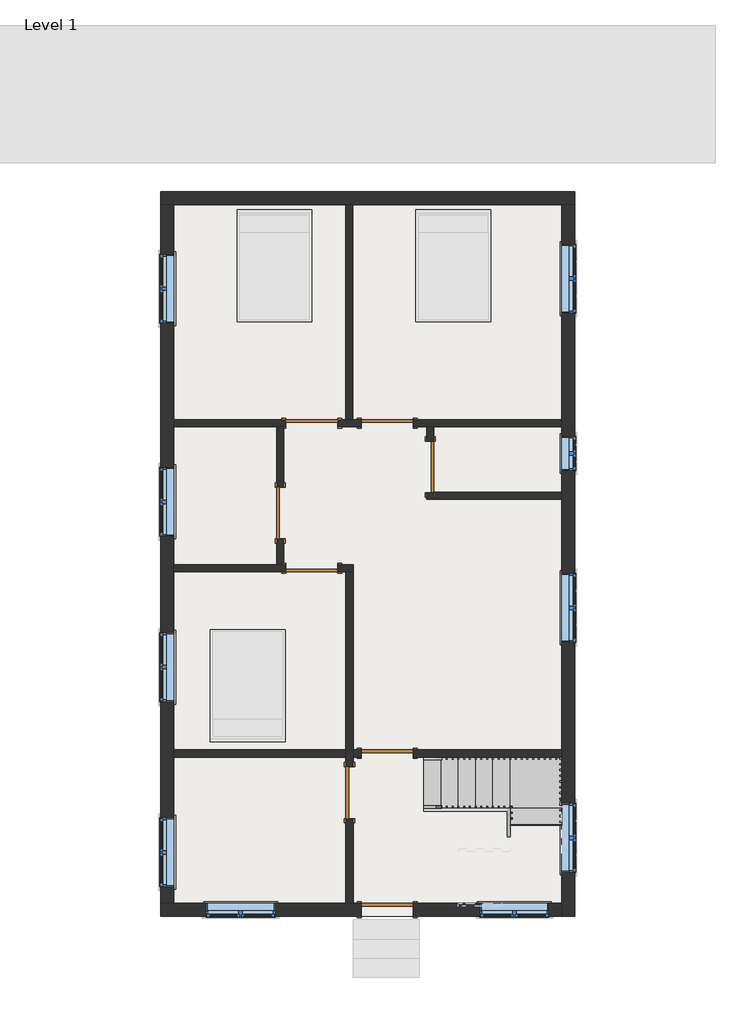
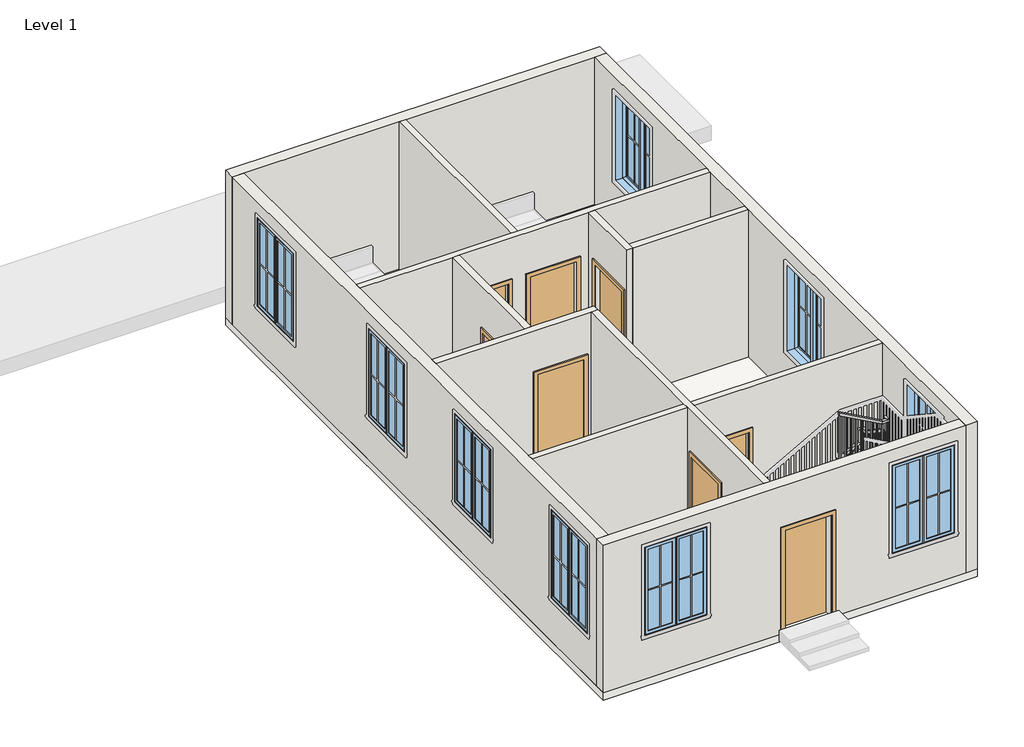
# One storey, part 1 of 2: 12 walls, 10 windows, 8 doors, 1 railing, 1 slab, 1 stair flight.
"""IFC4 building model written with IfcOpenShell, lengths in millimetres."""

from ifc_helpers import new_model, si_unit, frame, origin, origin_with_axes, place, context, project, spatial, polyline, outline, extrude, faceted_brep, transform, mapped, element, save
from components import door_a1797ceb, door_a3eb833a, door_a90ba1ad, stair_flight_16d52fd2, window_c417fced, window_6ca1769e

model = new_model("IFC4")

# Units and contexts
model_context = context("Model", 3, world=origin())
ifc_project = project(units=[si_unit("LENGTHUNIT", "METRE", prefix="MILLI")], contexts=[model_context])

# Site, building, storey
site = spatial("IfcSite", under=ifc_project)
building = spatial("IfcBuilding", under=site)
storey = spatial("IfcBuildingStorey", under=building, Name="Level 1", Elevation=0.0)

# Doors
placement = place(None, origin())
door_shape = door_a1797ceb(model_context)
element("IfcDoor", 1, ObjectType="Single-Flush : 36\" x 84\"", at=placement, inside=storey, context=model_context, shape_type="MappedRepresentation", body=[
    mapped(door_shape, transform((3683.0, 10363.2, 0.0), x_axis=(1.0, 0.0, 0.0), y_axis=(0.0, 1.0, 0.0), z_axis=(0.0, 0.0, 1.0))),
])
element("IfcDoor", 2, ObjectType="Single-Flush : 36\" x 84\"", at=placement, inside=storey, context=model_context, shape_type="MappedRepresentation", body=[
    mapped(door_shape, transform((3124.2, 8775.7, 0.0), x_axis=(0.0, 1.0, 0.0), y_axis=(-1.0, 0.0, 0.0), z_axis=(0.0, 0.0, 1.0))),
])
element("IfcDoor", 3, ObjectType="Single-Flush : 36\" x 84\"", at=placement, inside=storey, context=model_context, shape_type="MappedRepresentation", body=[
    mapped(door_shape, transform((3683.0, 7797.8, 0.0), x_axis=(-1.0, 0.0, 0.0), y_axis=(0.0, -1.0, 0.0), z_axis=(0.0, 0.0, 1.0))),
])
element("IfcDoor", 4, ObjectType="Single-Flush : 36\" x 84\"", at=placement, inside=storey, context=model_context, shape_type="MappedRepresentation", body=[
    mapped(door_shape, transform((4349.75, 3835.4, 0.0), x_axis=(0.0, 1.0, 0.0), y_axis=(-1.0, 0.0, 0.0), z_axis=(0.0, 0.0, 1.0))),
])
door_2_shape = door_a3eb833a(model_context)
element("IfcDoor", 5, ObjectType="Single-Flush : 36\" x 84\"", at=placement, inside=storey, context=model_context, shape_type="MappedRepresentation", body=[
    mapped(door_2_shape, transform((5016.5, 10363.2, 0.0), x_axis=(-1.0, 0.0, 0.0), y_axis=(0.0, -1.0, 0.0), z_axis=(0.0, 0.0, 1.0))),
])
element("IfcDoor", 6, ObjectType="Single-Flush : 36\" x 84\"", at=placement, inside=storey, context=model_context, shape_type="MappedRepresentation", body=[
    mapped(door_2_shape, transform((5778.5, 9588.5, 0.0), x_axis=(0.0, 1.0, 0.0), y_axis=(-1.0, 0.0, 0.0), z_axis=(0.0, 0.0, 1.0))),
])
element("IfcDoor", 7, ObjectType="Single-Flush : 36\" x 84\"", at=placement, inside=storey, context=model_context, shape_type="MappedRepresentation", body=[
    mapped(door_2_shape, transform((5016.5, 4527.55, 0.0), x_axis=(-1.0, 0.0, 0.0), y_axis=(0.0, -1.0, 0.0), z_axis=(0.0, 0.0, 1.0))),
])
door_3_shape = door_a90ba1ad(model_context)
element("IfcDoor", 8, ObjectType="Single-Flush : 36\" x 84\"", at=placement, inside=storey, context=model_context, shape_type="MappedRepresentation", body=[
    mapped(door_3_shape, transform((5016.5, 1765.3, 0.0), x_axis=(-1.0, 0.0, 0.0), y_axis=(0.0, -1.0, 0.0), z_axis=(0.0, 0.0, 1.0))),
])

# Railing
element("IfcRailing", 9, ObjectType="Handrail - Rectangular", at=placement, inside=storey, context=model_context, shape_type="SolidModel", body=[
    faceted_brep([(5664.2, 3606.8, 1083.7333333), (5664.2, 3606.8, 1025.620221), (5664.2, 3556.0, 1025.620221), (5664.2, 3556.0, 1083.7333333), (7112.0, 3606.8, 1888.0666667), (7162.8, 3606.8, 1858.1757765), (7162.8, 3556.0, 1858.1757765), (7112.0, 3556.0, 1888.0666667), (7112.0, 3606.8, 2150.5333333), (7162.8, 3606.8, 2099.7333333), (7162.8, 3556.0, 2099.7333333), (7112.0, 3556.0, 2150.5333333), (7239.0, 3606.8, 2150.5333333), (7239.0, 3606.8, 2099.7333333), (7188.2, 3556.0, 2099.7333333), (7188.2, 3556.0, 2150.5333333), (7239.0, 3479.8, 2150.5333333), (7239.0, 3464.4189976, 2099.7333333), (7188.2, 3464.4189976, 2099.7333333), (7188.2, 3479.8, 2150.5333333), (7239.0, 2870.2, 2556.9333333), (7239.0, 2819.4, 2529.7459984), (7188.2, 2819.4, 2529.7459984), (7188.2, 2870.2, 2556.9333333), (7239.0, 2870.2, 2819.3694921), (7239.0, 2819.4, 2768.5694921), (7188.2, 2819.4, 2768.5694921), (7188.2, 2870.2, 2819.3694921), (7239.0, 2743.2, 2819.3694921), (7239.0, 2743.2, 2768.5694921), (7188.2, 2794.0, 2768.5694921), (7188.2, 2794.0, 2819.3694921), (7112.0, 2743.2, 2819.3694921), (7098.8446915, 2743.2, 2768.5694921), (7098.8446915, 2794.0, 2768.5694921), (7112.0, 2794.0, 2819.3694921), (6273.1405542, 2743.2, 3285.0666667), (6273.1405542, 2794.0, 3285.0666667), (6273.1405542, 2794.0, 3226.9634289), (6273.1405542, 2743.2, 3226.9634289)], [[[0, 1, 2, 3]], [[1, 0, 4, 5]], [[2, 1, 5, 6]], [[3, 2, 6, 7]], [[0, 3, 7, 4]], [[5, 4, 8, 9]], [[6, 5, 9, 10]], [[7, 6, 10, 11]], [[4, 7, 11, 8]], [[9, 8, 12, 13]], [[10, 9, 13, 14]], [[11, 10, 14, 15]], [[8, 11, 15, 12]], [[13, 12, 16, 17]], [[14, 13, 17, 18]], [[15, 14, 18, 19]], [[12, 15, 19, 16]], [[17, 16, 20, 21]], [[18, 17, 21, 22]], [[19, 18, 22, 23]], [[16, 19, 23, 20]], [[21, 20, 24, 25]], [[22, 21, 25, 26]], [[23, 22, 26, 27]], [[20, 23, 27, 24]], [[25, 24, 28, 29]], [[26, 25, 29, 30]], [[27, 26, 30, 31]], [[24, 27, 31, 28]], [[29, 28, 32, 33]], [[30, 29, 33, 34]], [[31, 30, 34, 35]], [[28, 31, 35, 32]], [[36, 37, 38, 39]], [[33, 32, 36, 39]], [[34, 33, 39, 38]], [[35, 34, 38, 37]], [[32, 35, 37, 36]]]),
    extrude(outline(polyline([(3207.2085391, 6308.725), (3217.7842455, 6289.675), (2201.3333333, 6289.675), (2201.3333333, 6308.725), (3207.2085391, 6308.725)])), frame((0.0, 2759.075, 0.0), z_axis=(0.0, 1.0, 0.0), x_axis=(0.0, 0.0, 1.0)), (0.0, 0.0, 1.0), 19.05),
    extrude(outline(polyline([(3150.8047719, 6410.325), (3161.3804782, 6391.275), (2201.3333333, 6391.275), (2201.3333333, 6410.325), (3150.8047719, 6410.325)])), frame((0.0, 2759.075, 0.0), z_axis=(0.0, 1.0, 0.0), x_axis=(0.0, 0.0, 1.0)), (0.0, 0.0, 1.0), 19.05),
    extrude(outline(polyline([(3094.4010046, 6511.925), (3104.976711, 6492.875), (2201.3333333, 6492.875), (2201.3333333, 6511.925), (3094.4010046, 6511.925)])), frame((0.0, 2759.075, 0.0), z_axis=(0.0, 1.0, 0.0), x_axis=(0.0, 0.0, 1.0)), (0.0, 0.0, 1.0), 19.05),
    extrude(outline(polyline([(3037.8752058, 6613.525), (3048.4509122, 6594.475), (2032.0, 6594.475), (2032.0, 6613.525), (3037.8752058, 6613.525)])), frame((0.0, 2759.075, 0.0), z_axis=(0.0, 1.0, 0.0), x_axis=(0.0, 0.0, 1.0)), (0.0, 0.0, 1.0), 19.05),
    extrude(outline(polyline([(2981.4714386, 6715.125), (2992.0471449, 6696.075), (2032.0, 6696.075), (2032.0, 6715.125), (2981.4714386, 6715.125)])), frame((0.0, 2759.075, 0.0), z_axis=(0.0, 1.0, 0.0), x_axis=(0.0, 0.0, 1.0)), (0.0, 0.0, 1.0), 19.05),
    extrude(outline(polyline([(2925.0676713, 6816.725), (2935.6433777, 6797.675), (2032.0, 6797.675), (2032.0, 6816.725), (2925.0676713, 6816.725)])), frame((0.0, 2759.075, 0.0), z_axis=(0.0, 1.0, 0.0), x_axis=(0.0, 0.0, 1.0)), (0.0, 0.0, 1.0), 19.05),
    extrude(outline(polyline([(2868.7859356, 6918.325), (2879.361642, 6899.275), (1862.6666667, 6899.275), (1862.6666667, 6918.325), (2868.7859356, 6918.325)])), frame((0.0, 2759.075, 0.0), z_axis=(0.0, 1.0, 0.0), x_axis=(0.0, 0.0, 1.0)), (0.0, 0.0, 1.0), 19.05),
    extrude(outline(polyline([(2812.3821684, 7019.925), (2822.9578748, 7000.875), (1862.6666667, 7000.875), (1862.6666667, 7019.925), (2812.3821684, 7019.925)])), frame((0.0, 2759.075, 0.0), z_axis=(0.0, 1.0, 0.0), x_axis=(0.0, 0.0, 1.0)), (0.0, 0.0, 1.0), 19.05),
    extrude(outline(polyline([(2755.9784011, 7121.525), (2766.5541075, 7102.475), (1862.6666667, 7102.475), (1862.6666667, 7121.525), (2755.9784011, 7121.525)])), frame((0.0, 2759.075, 0.0), z_axis=(0.0, 1.0, 0.0), x_axis=(0.0, 0.0, 1.0)), (0.0, 0.0, 1.0), 19.05),
    extrude(outline(polyline([(2860.675, 2502.2293317), (2879.725, 2489.5293317), (2879.725, 1524.0), (2860.675, 1524.0), (2860.675, 2502.2293317)])), frame((7204.075, 0.0, 0.0), z_axis=(1.0, 0.0, 0.0), x_axis=(0.0, 1.0, 0.0)), (0.0, 0.0, 1.0), 19.05),
    extrude(outline(polyline([(2962.275, 2434.4959984), (2981.325, 2421.7959984), (2981.325, 1524.0), (2962.275, 1524.0), (2962.275, 2434.4959984)])), frame((7204.075, 0.0, 0.0), z_axis=(1.0, 0.0, 0.0), x_axis=(0.0, 1.0, 0.0)), (0.0, 0.0, 1.0), 19.05),
    extrude(outline(polyline([(3063.875, 2366.7626651), (3082.925, 2354.0626651), (3082.925, 1354.6666667), (3063.875, 1354.6666667), (3063.875, 2366.7626651)])), frame((7204.075, 0.0, 0.0), z_axis=(1.0, 0.0, 0.0), x_axis=(0.0, 1.0, 0.0)), (0.0, 0.0, 1.0), 19.05),
    extrude(outline(polyline([(3165.475, 2299.0293317), (3184.525, 2286.3293317), (3184.525, 1354.6666667), (3165.475, 1354.6666667), (3165.475, 2299.0293317)])), frame((7204.075, 0.0, 0.0), z_axis=(1.0, 0.0, 0.0), x_axis=(0.0, 1.0, 0.0)), (0.0, 0.0, 1.0), 19.05),
    extrude(outline(polyline([(3267.075, 2231.2959984), (3286.125, 2218.5959984), (3286.125, 1354.6666667), (3267.075, 1354.6666667), (3267.075, 2231.2959984)])), frame((7204.075, 0.0, 0.0), z_axis=(1.0, 0.0, 0.0), x_axis=(0.0, 1.0, 0.0)), (0.0, 0.0, 1.0), 19.05),
    extrude(outline(polyline([(3368.675, 2163.5626651), (3387.725, 2150.8626651), (3387.725, 1185.3333333), (3368.675, 1185.3333333), (3368.675, 2163.5626651)])), frame((7204.075, 0.0, 0.0), z_axis=(1.0, 0.0, 0.0), x_axis=(0.0, 1.0, 0.0)), (0.0, 0.0, 1.0), 19.05),
    extrude(outline(polyline([(3470.275, 2095.8293317), (3489.325, 2083.1293317), (3489.325, 1185.3333333), (3470.275, 1185.3333333), (3470.275, 2095.8293317)])), frame((7204.075, 0.0, 0.0), z_axis=(1.0, 0.0, 0.0), x_axis=(0.0, 1.0, 0.0)), (0.0, 0.0, 1.0), 19.05),
    extrude(outline(polyline([(7178.675, 3571.875), (7178.675, 3590.925), (7197.725, 3590.925), (7197.725, 3571.875), (7178.675, 3571.875)])), frame((0.0, 0.0, 1016.0), z_axis=(0.0, 0.0, 1.0), x_axis=(1.0, 0.0, 0.0)), (0.0, 0.0, 1.0), 1083.7333333),
    extrude(outline(polyline([(1821.1341099, 7096.125), (1810.5507765, 7077.075), (846.6666667, 7077.075), (846.6666667, 7096.125), (1821.1341099, 7096.125)])), frame((0.0, 3571.875, 0.0), z_axis=(0.0, 1.0, 0.0), x_axis=(0.0, 0.0, 1.0)), (0.0, 0.0, 1.0), 19.05),
    extrude(outline(polyline([(1764.6896654, 6994.525), (1754.1063321, 6975.475), (846.6666667, 6975.475), (846.6666667, 6994.525), (1764.6896654, 6994.525)])), frame((0.0, 3571.875, 0.0), z_axis=(0.0, 1.0, 0.0), x_axis=(0.0, 0.0, 1.0)), (0.0, 0.0, 1.0), 19.05),
    extrude(outline(polyline([(1708.245221, 6892.925), (1697.6618876, 6873.875), (846.6666667, 6873.875), (846.6666667, 6892.925), (1708.245221, 6892.925)])), frame((0.0, 3571.875, 0.0), z_axis=(0.0, 1.0, 0.0), x_axis=(0.0, 0.0, 1.0)), (0.0, 0.0, 1.0), 19.05),
    extrude(outline(polyline([(1651.8007765, 6791.325), (1641.2174432, 6772.275), (677.3333333, 6772.275), (677.3333333, 6791.325), (1651.8007765, 6791.325)])), frame((0.0, 3571.875, 0.0), z_axis=(0.0, 1.0, 0.0), x_axis=(0.0, 0.0, 1.0)), (0.0, 0.0, 1.0), 19.05),
    extrude(outline(polyline([(1595.3563321, 6689.725), (1584.7729988, 6670.675), (677.3333333, 6670.675), (677.3333333, 6689.725), (1595.3563321, 6689.725)])), frame((0.0, 3571.875, 0.0), z_axis=(0.0, 1.0, 0.0), x_axis=(0.0, 0.0, 1.0)), (0.0, 0.0, 1.0), 19.05),
    extrude(outline(polyline([(1538.9118876, 6588.125), (1528.3285543, 6569.075), (677.3333333, 6569.075), (677.3333333, 6588.125), (1538.9118876, 6588.125)])), frame((0.0, 3571.875, 0.0), z_axis=(0.0, 1.0, 0.0), x_axis=(0.0, 0.0, 1.0)), (0.0, 0.0, 1.0), 19.05),
    extrude(outline(polyline([(1482.4674432, 6486.525), (1471.8841099, 6467.475), (508.0, 6467.475), (508.0, 6486.525), (1482.4674432, 6486.525)])), frame((0.0, 3571.875, 0.0), z_axis=(0.0, 1.0, 0.0), x_axis=(0.0, 0.0, 1.0)), (0.0, 0.0, 1.0), 19.05),
    extrude(outline(polyline([(1426.0229988, 6384.925), (1415.4396654, 6365.875), (508.0, 6365.875), (508.0, 6384.925), (1426.0229988, 6384.925)])), frame((0.0, 3571.875, 0.0), z_axis=(0.0, 1.0, 0.0), x_axis=(0.0, 0.0, 1.0)), (0.0, 0.0, 1.0), 19.05),
    extrude(outline(polyline([(1369.5785543, 6283.325), (1358.995221, 6264.275), (508.0, 6264.275), (508.0, 6283.325), (1369.5785543, 6283.325)])), frame((0.0, 3571.875, 0.0), z_axis=(0.0, 1.0, 0.0), x_axis=(0.0, 0.0, 1.0)), (0.0, 0.0, 1.0), 19.05),
    extrude(outline(polyline([(1313.1341099, 6181.725), (1302.5507765, 6162.675), (338.6666667, 6162.675), (338.6666667, 6181.725), (1313.1341099, 6181.725)])), frame((0.0, 3571.875, 0.0), z_axis=(0.0, 1.0, 0.0), x_axis=(0.0, 0.0, 1.0)), (0.0, 0.0, 1.0), 19.05),
    extrude(outline(polyline([(1256.6896654, 6080.125), (1246.1063321, 6061.075), (338.6666667, 6061.075), (338.6666667, 6080.125), (1256.6896654, 6080.125)])), frame((0.0, 3571.875, 0.0), z_axis=(0.0, 1.0, 0.0), x_axis=(0.0, 0.0, 1.0)), (0.0, 0.0, 1.0), 19.05),
    extrude(outline(polyline([(1200.245221, 5978.525), (1189.6618876, 5959.475), (338.6666667, 5959.475), (338.6666667, 5978.525), (1200.245221, 5978.525)])), frame((0.0, 3571.875, 0.0), z_axis=(0.0, 1.0, 0.0), x_axis=(0.0, 0.0, 1.0)), (0.0, 0.0, 1.0), 19.05),
    extrude(outline(polyline([(1143.8007765, 5876.925), (1133.2174432, 5857.875), (169.3333333, 5857.875), (169.3333333, 5876.925), (1143.8007765, 5876.925)])), frame((0.0, 3571.875, 0.0), z_axis=(0.0, 1.0, 0.0), x_axis=(0.0, 0.0, 1.0)), (0.0, 0.0, 1.0), 19.05),
    extrude(outline(polyline([(1087.3563321, 5775.325), (1076.7729988, 5756.275), (169.3333333, 5756.275), (169.3333333, 5775.325), (1087.3563321, 5775.325)])), frame((0.0, 3571.875, 0.0), z_axis=(0.0, 1.0, 0.0), x_axis=(0.0, 0.0, 1.0)), (0.0, 0.0, 1.0), 19.05),
    extrude(outline(polyline([(7204.075, 2778.125), (7223.125, 2778.125), (7223.125, 2759.075), (7204.075, 2759.075), (7204.075, 2778.125)])), frame((0.0, 0.0, 1693.3333333), z_axis=(0.0, 0.0, 1.0), x_axis=(1.0, 0.0, 0.0)), (0.0, 0.0, 1.0), 1075.2361588),
    extrude(outline(polyline([(7204.075, 3571.875), (7204.075, 3590.925), (7223.125, 3590.925), (7223.125, 3571.875), (7204.075, 3571.875)])), frame((0.0, 0.0, 1016.0), z_axis=(0.0, 0.0, 1.0), x_axis=(1.0, 0.0, 0.0)), (0.0, 0.0, 1.0), 1083.7333333),
    extrude(outline(polyline([(3216.3877225, 6292.1905542), (3226.9634289, 6273.1405542), (2201.3333333, 6273.1405542), (2201.3333333, 6292.1905542), (3216.3877225, 6292.1905542)])), frame((0.0, 2759.075, 0.0), z_axis=(0.0, 1.0, 0.0), x_axis=(0.0, 0.0, 1.0)), (0.0, 0.0, 1.0), 19.05),
    extrude(outline(polyline([(1036.2035543, 5683.25), (1025.620221, 5664.2), (169.3333333, 5664.2), (169.3333333, 5683.25), (1036.2035543, 5683.25)])), frame((0.0, 3571.875, 0.0), z_axis=(0.0, 1.0, 0.0), x_axis=(0.0, 0.0, 1.0)), (0.0, 0.0, 1.0), 19.05),
])

# Slab
element("IfcSlab", 10, ObjectType="Generic - 12\"", at=placement, inside=storey, context=model_context, shape_type="SweptSolid", body=[
    extrude(outline(polyline([(8331.2, 14452.6), (8331.2, 1651.0), (1016.0, 1651.0), (1016.0, 14452.6), (8331.2, 14452.6)])), frame((0.0, 0.0, -152.4), z_axis=(0.0, 0.0, 1.0), x_axis=(1.0, 0.0, 0.0)), (0.0, 0.0, 1.0), 152.4),
])

# Stair flight
stair_flight_shape = stair_flight_16d52fd2(model_context)
element("IfcStairFlight", 11, ObjectType="2\" Tread 1\" Nosing 1/4\" Riser", at=placement, inside=storey, context=model_context, shape_type="MappedRepresentation", body=[
    mapped(stair_flight_shape, transform((0.0, 0.0, 0.0), x_axis=(1.0, 0.0, 0.0), y_axis=(0.0, 1.0, 0.0), z_axis=(0.0, 0.0, 1.0))),
])

# Walls
element("IfcWall", 12, ObjectType="Generic - 5\"", at=placement, inside=storey, context=model_context, shape_type="SweptSolid", body=[
    extrude(outline(polyline([(4279.9, 10426.7), (4279.9, 14224.0), (4406.9, 14224.0), (4406.9, 10426.7), (4279.9, 10426.7)])), origin_with_axes(), (0.0, 0.0, 1.0), 3048.0),
])
element("IfcWall", 13, ObjectType="Generic - 5\"", at=placement, inside=storey, context=model_context, shape_type="Brep", body=[
    faceted_brep([(4140.2, 10299.7, 0.0), (4559.3, 10299.7, 0.0), (4559.3, 10299.7, 2133.6), (5473.7, 10299.7, 2133.6), (5473.7, 10299.7, 0.0), (5715.0, 10299.7, 0.0), (5842.0, 10299.7, 0.0), (8102.6, 10299.7, 0.0), (8102.6, 10299.7, 3048.0), (5842.0, 10299.7, 3048.0), (5715.0, 10299.7, 3048.0), (3187.7, 10299.7, 3048.0), (3060.7, 10299.7, 3048.0), (1244.6, 10299.7, 3048.0), (1244.6, 10299.7, 0.0), (3060.7, 10299.7, 0.0), (3187.7, 10299.7, 0.0), (3225.8, 10299.7, 0.0), (3225.8, 10299.7, 2133.6), (4140.2, 10299.7, 2133.6), (4559.3, 10426.7, 2133.6), (4559.3, 10426.7, 0.0), (4406.9, 10426.7, 0.0), (4279.9, 10426.7, 0.0), (4140.2, 10426.7, 0.0), (4140.2, 10426.7, 2133.6), (3225.8, 10426.7, 2133.6), (3225.8, 10426.7, 0.0), (1244.6, 10426.7, 0.0), (1244.6, 10426.7, 3048.0), (4279.9, 10426.7, 3048.0), (4406.9, 10426.7, 3048.0), (8102.6, 10426.7, 3048.0), (8102.6, 10426.7, 0.0), (5473.7, 10426.7, 0.0), (5473.7, 10426.7, 2133.6)], [[[0, 1, 2, 3, 4, 5, 6, 7, 8, 9, 10, 11, 12, 13, 14, 15, 16, 17, 18, 19]], [[20, 21, 22, 23, 24, 25, 26, 27, 28, 29, 30, 31, 32, 33, 34, 35]], [[17, 16, 15, 14, 28, 27]], [[34, 33, 7, 6, 5, 4]], [[24, 23, 22, 21, 1, 0]], [[13, 12, 11, 10, 9, 8, 32, 31, 30, 29]], [[8, 7, 33, 32]], [[14, 13, 29, 28]], [[25, 24, 0, 19]], [[26, 25, 19, 18]], [[27, 26, 18, 17]], [[2, 1, 21, 20]], [[3, 2, 20, 35]], [[4, 3, 35, 34]]]),
])
element("IfcWall", 14, ObjectType="Generic - 5\"", at=placement, inside=storey, context=model_context, shape_type="Brep", body=[
    faceted_brep([(1244.6, 7734.3, 0.0), (3225.8, 7734.3, 0.0), (3225.8, 7734.3, 2133.6), (4140.2, 7734.3, 2133.6), (4140.2, 7734.3, 0.0), (4286.25, 7734.3, 0.0), (4413.25, 7734.3, 0.0), (4413.25, 7734.3, 3048.0), (4286.25, 7734.3, 3048.0), (1244.6, 7734.3, 3048.0), (3225.8, 7861.3, 2133.6), (3225.8, 7861.3, 0.0), (3187.7, 7861.3, 0.0), (3060.7, 7861.3, 0.0), (1244.6, 7861.3, 0.0), (1244.6, 7861.3, 3048.0), (3060.7, 7861.3, 3048.0), (3187.7, 7861.3, 3048.0), (4413.25, 7861.3, 3048.0), (4413.25, 7861.3, 0.0), (4140.2, 7861.3, 0.0), (4140.2, 7861.3, 2133.6)], [[[0, 1, 2, 3, 4, 5, 6, 7, 8, 9]], [[10, 11, 12, 13, 14, 15, 16, 17, 18, 19, 20, 21]], [[20, 19, 6, 5, 4]], [[14, 13, 12, 11, 1, 0]], [[9, 8, 7, 18, 17, 16, 15]], [[0, 9, 15, 14]], [[7, 6, 19, 18]], [[2, 1, 11, 10]], [[3, 2, 10, 21]], [[4, 3, 21, 20]]]),
])
element("IfcWall", 15, ObjectType="Generic - 5\"", at=placement, inside=storey, context=model_context, shape_type="SweptSolid", body=[
    extrude(outline(polyline([(10299.7, 0.0), (9232.9, 0.0), (9232.9, 2133.6), (8318.5, 2133.6), (8318.5, 0.0), (7861.3, 0.0), (7861.3, 3048.0), (10299.7, 3048.0), (10299.7, 0.0)])), frame((3060.7, 0.0, 0.0), z_axis=(1.0, 0.0, 0.0), x_axis=(0.0, 1.0, 0.0)), (0.0, 0.0, 1.0), 127.0),
])
element("IfcWall", 16, ObjectType="Generic - 5\"", at=placement, inside=storey, context=model_context, shape_type="Brep", body=[
    faceted_brep([(5715.0, 10299.7, 0.0), (5715.0, 10045.7, 0.0), (5715.0, 10045.7, 2133.6), (5715.0, 9131.3, 2133.6), (5715.0, 9131.3, 0.0), (5715.0, 9017.0, 0.0), (5715.0, 9017.0, 3048.0), (5715.0, 10299.7, 3048.0), (5842.0, 10045.7, 2133.6), (5842.0, 10045.7, 0.0), (5842.0, 10299.7, 0.0), (5842.0, 10299.7, 3048.0), (5842.0, 9144.0, 3048.0), (5842.0, 9017.0, 3048.0), (5842.0, 9017.0, 0.0), (5842.0, 9131.3, 0.0), (5842.0, 9131.3, 2133.6)], [[[0, 1, 2, 3, 4, 5, 6, 7]], [[8, 9, 10, 11, 12, 13, 14, 15, 16]], [[10, 9, 1, 0]], [[15, 14, 5, 4]], [[7, 6, 13, 12, 11]], [[0, 7, 11, 10]], [[6, 5, 14, 13]], [[2, 1, 9, 8]], [[3, 2, 8, 16]], [[4, 3, 16, 15]]]),
])
element("IfcWall", 17, ObjectType="Generic - 5\"", at=placement, inside=storey, context=model_context, shape_type="Brep", body=[
    faceted_brep([(5842.0, 9017.0, 0.0), (8102.6, 9017.0, 0.0), (8102.6, 9017.0, 3048.0), (5842.0, 9017.0, 3048.0), (5842.0, 9144.0, 0.0), (5842.0, 9144.0, 3048.0), (8102.6, 9144.0, 3048.0), (8102.6, 9144.0, 0.0), (5842.0, 9131.3, 0.0)], [[[0, 1, 2, 3]], [[4, 5, 6, 7]], [[1, 0, 8, 4, 7]], [[3, 2, 6, 5]], [[0, 3, 5, 4, 8]], [[2, 1, 7, 6]]]),
])
element("IfcWall", 18, ObjectType="Generic - 5\"", at=placement, inside=storey, context=model_context, shape_type="Brep", body=[
    faceted_brep([(4286.25, 7734.3, 0.0), (4286.25, 4591.05, 0.0), (4286.25, 4464.05, 0.0), (4286.25, 4292.6, 0.0), (4286.25, 4292.6, 2133.6), (4286.25, 3378.2, 2133.6), (4286.25, 3378.2, 0.0), (4286.25, 1879.6, 0.0), (4286.25, 1879.6, 3048.0), (4286.25, 4464.05, 3048.0), (4286.25, 4591.05, 3048.0), (4286.25, 7734.3, 3048.0), (4413.25, 4292.6, 2133.6), (4413.25, 4292.6, 0.0), (4413.25, 4464.05, 0.0), (4413.25, 4591.05, 0.0), (4413.25, 7734.3, 0.0), (4413.25, 7734.3, 3048.0), (4413.25, 4591.05, 3048.0), (4413.25, 4464.05, 3048.0), (4413.25, 1879.6, 3048.0), (4413.25, 1879.6, 0.0), (4413.25, 3378.2, 0.0), (4413.25, 3378.2, 2133.6)], [[[0, 1, 2, 3, 4, 5, 6, 7, 8, 9, 10, 11]], [[12, 13, 14, 15, 16, 17, 18, 19, 20, 21, 22, 23]], [[22, 21, 7, 6]], [[16, 15, 14, 13, 3, 2, 1, 0]], [[11, 10, 9, 8, 20, 19, 18, 17]], [[0, 11, 17, 16]], [[8, 7, 21, 20]], [[4, 3, 13, 12]], [[5, 4, 12, 23]], [[6, 5, 23, 22]]]),
])
element("IfcWall", 19, ObjectType="Generic - 5\"", at=placement, inside=storey, context=model_context, shape_type="SweptSolid", body=[
    extrude(outline(polyline([(0.0, 8102.6), (3048.0, 8102.6), (3048.0, 4413.25), (0.0, 4413.25), (0.0, 4559.3), (2133.6, 4559.3), (2133.6, 5473.7), (0.0, 5473.7), (0.0, 8102.6)])), frame((0.0, 4464.05, 0.0), z_axis=(0.0, 1.0, 0.0), x_axis=(0.0, 0.0, 1.0)), (0.0, 0.0, 1.0), 127.0),
    extrude(outline(polyline([(1244.6, 4464.05), (1244.6, 4591.05), (4286.25, 4591.05), (4286.25, 4464.05), (1244.6, 4464.05)])), origin_with_axes(), (0.0, 0.0, 1.0), 3048.0),
])
element("IfcWall", 20, ObjectType="Generic - 8\"", at=placement, inside=storey, context=model_context, shape_type="Brep", body=[
    faceted_brep([(1016.0, 14224.0, 0.0), (1244.6, 14224.0, 0.0), (4279.9, 14224.0, 0.0), (4406.9, 14224.0, 0.0), (8102.6, 14224.0, 0.0), (8331.2, 14224.0, 0.0), (8331.2, 14224.0, 3048.0), (8102.6, 14224.0, 3048.0), (4406.9, 14224.0, 3048.0), (4279.9, 14224.0, 3048.0), (1244.6, 14224.0, 3048.0), (1016.0, 14224.0, 3048.0), (1016.0, 14452.6, 0.0), (1016.0, 14452.6, 3048.0), (8331.2, 14452.6, 3048.0), (8331.2, 14452.6, 0.0)], [[[0, 1, 2, 3, 4, 5, 6, 7, 8, 9, 10, 11]], [[12, 13, 14, 15]], [[5, 4, 3, 2, 1, 0, 12, 15]], [[6, 5, 15, 14]], [[0, 11, 13, 12]], [[11, 10, 9, 8, 7, 6, 14, 13]]]),
])
element("IfcWall", 21, ObjectType="Generic - 8\"", at=placement, inside=storey, context=model_context, shape_type="Brep", body=[
    faceted_brep([(8102.6, 14224.0, 0.0), (8102.6, 10426.7, 0.0), (8102.6, 10299.7, 0.0), (8102.6, 9144.0, 0.0), (8102.6, 9017.0, 0.0), (8102.6, 4591.05, 0.0), (8102.6, 4464.05, 0.0), (8102.6, 1879.6, 0.0), (8102.6, 1651.0, 0.0), (8102.6, 1651.0, 3048.0), (8102.6, 1879.6, 3048.0), (8102.6, 4464.05, 3048.0), (8102.6, 4591.05, 3048.0), (8102.6, 9017.0, 3048.0), (8102.6, 9144.0, 3048.0), (8102.6, 10299.7, 3048.0), (8102.6, 10426.7, 3048.0), (8102.6, 14224.0, 3048.0), (8102.6, 12306.3, 2743.2), (8102.6, 12306.3, 914.4), (8102.6, 13525.5, 914.4), (8102.6, 13525.5, 2743.2), (8102.6, 2425.7, 2743.2), (8102.6, 2425.7, 914.4), (8102.6, 3644.9, 914.4), (8102.6, 3644.9, 2743.2), (8102.6, 6489.7, 2743.2), (8102.6, 6489.7, 914.4), (8102.6, 7708.9, 914.4), (8102.6, 7708.9, 2743.2), (8102.6, 9525.0, 1828.8), (8102.6, 9525.0, 914.4), (8102.6, 10134.6, 914.4), (8102.6, 10134.6, 1828.8), (8331.2, 14224.0, 0.0), (8331.2, 14224.0, 3048.0), (8331.2, 1651.0, 3048.0), (8331.2, 1651.0, 0.0), (8331.2, 12306.3, 2743.2), (8331.2, 13525.5, 2743.2), (8331.2, 13525.5, 914.4), (8331.2, 12306.3, 914.4), (8331.2, 2425.7, 2743.2), (8331.2, 3644.9, 2743.2), (8331.2, 3644.9, 914.4), (8331.2, 2425.7, 914.4), (8331.2, 6489.7, 2743.2), (8331.2, 7708.9, 2743.2), (8331.2, 7708.9, 914.4), (8331.2, 6489.7, 914.4), (8331.2, 9525.0, 1828.8), (8331.2, 10134.6, 1828.8), (8331.2, 10134.6, 914.4), (8331.2, 9525.0, 914.4)], [[[0, 1, 2, 3, 4, 5, 6, 7, 8, 9, 10, 11, 12, 13, 14, 15, 16, 17], [18, 19, 20, 21], [22, 23, 24, 25], [26, 27, 28, 29], [30, 31, 32, 33]], [[34, 35, 36, 37], [38, 39, 40, 41], [42, 43, 44, 45], [46, 47, 48, 49], [50, 51, 52, 53]], [[8, 7, 6, 5, 4, 3, 2, 1, 0, 34, 37]], [[0, 17, 35, 34]], [[9, 8, 37, 36]], [[19, 18, 38, 41]], [[20, 19, 41, 40]], [[21, 20, 40, 39]], [[18, 21, 39, 38]], [[23, 22, 42, 45]], [[24, 23, 45, 44]], [[25, 24, 44, 43]], [[22, 25, 43, 42]], [[27, 26, 46, 49]], [[28, 27, 49, 48]], [[29, 28, 48, 47]], [[26, 29, 47, 46]], [[31, 30, 50, 53]], [[32, 31, 53, 52]], [[33, 32, 52, 51]], [[30, 33, 51, 50]], [[17, 16, 15, 14, 13, 12, 11, 10, 9, 36, 35]]]),
])
element("IfcWall", 22, ObjectType="Generic - 8\"", at=placement, inside=storey, context=model_context, shape_type="Brep", body=[
    faceted_brep([(4559.3, 1879.6, 2133.6), (4559.3, 1879.6, 0.0), (4413.25, 1879.6, 0.0), (4286.25, 1879.6, 0.0), (1244.6, 1879.6, 0.0), (1016.0, 1879.6, 0.0), (1016.0, 1879.6, 3048.0), (1244.6, 1879.6, 3048.0), (4286.25, 1879.6, 3048.0), (4413.25, 1879.6, 3048.0), (8102.6, 1879.6, 3048.0), (8102.6, 1879.6, 0.0), (5473.7, 1879.6, 0.0), (5473.7, 1879.6, 2133.6), (6654.8, 1879.6, 2743.2), (6654.8, 1879.6, 914.4), (7874.0, 1879.6, 914.4), (7874.0, 1879.6, 2743.2), (1816.1, 1879.6, 2743.2), (1816.1, 1879.6, 914.4), (3035.3, 1879.6, 914.4), (3035.3, 1879.6, 2743.2), (1016.0, 1651.0, 0.0), (4559.3, 1651.0, 0.0), (4559.3, 1651.0, 2133.6), (5473.7, 1651.0, 2133.6), (5473.7, 1651.0, 0.0), (8102.6, 1651.0, 0.0), (8102.6, 1651.0, 3048.0), (1016.0, 1651.0, 3048.0), (6654.8, 1651.0, 2743.2), (7874.0, 1651.0, 2743.2), (7874.0, 1651.0, 914.4), (6654.8, 1651.0, 914.4), (1816.1, 1651.0, 2743.2), (3035.3, 1651.0, 2743.2), (3035.3, 1651.0, 914.4), (1816.1, 1651.0, 914.4)], [[[0, 1, 2, 3, 4, 5, 6, 7, 8, 9, 10, 11, 12, 13], [14, 15, 16, 17], [18, 19, 20, 21]], [[22, 23, 24, 25, 26, 27, 28, 29], [30, 31, 32, 33], [34, 35, 36, 37]], [[12, 11, 27, 26]], [[5, 4, 3, 2, 1, 23, 22]], [[11, 10, 28, 27]], [[6, 5, 22, 29]], [[24, 23, 1, 0]], [[25, 24, 0, 13]], [[26, 25, 13, 12]], [[15, 14, 30, 33]], [[16, 15, 33, 32]], [[17, 16, 32, 31]], [[14, 17, 31, 30]], [[19, 18, 34, 37]], [[20, 19, 37, 36]], [[21, 20, 36, 35]], [[18, 21, 35, 34]], [[10, 9, 8, 7, 6, 29, 28]]]),
])
element("IfcWall", 23, ObjectType="Generic - 8\"", at=placement, inside=storey, context=model_context, shape_type="Brep", body=[
    faceted_brep([(1244.6, 1879.6, 0.0), (1244.6, 4464.05, 0.0), (1244.6, 4591.05, 0.0), (1244.6, 7734.3, 0.0), (1244.6, 7861.3, 0.0), (1244.6, 10299.7, 0.0), (1244.6, 10426.7, 0.0), (1244.6, 14224.0, 0.0), (1244.6, 14224.0, 3048.0), (1244.6, 10426.7, 3048.0), (1244.6, 10299.7, 3048.0), (1244.6, 7861.3, 3048.0), (1244.6, 7734.3, 3048.0), (1244.6, 4591.05, 3048.0), (1244.6, 4464.05, 3048.0), (1244.6, 1879.6, 3048.0), (1244.6, 13347.7, 2743.2), (1244.6, 13347.7, 914.4), (1244.6, 12128.5, 914.4), (1244.6, 12128.5, 2743.2), (1244.6, 3390.9, 2743.2), (1244.6, 3390.9, 914.4), (1244.6, 2171.7, 914.4), (1244.6, 2171.7, 2743.2), (1244.6, 6661.15, 2743.2), (1244.6, 6661.15, 914.4), (1244.6, 5441.95, 914.4), (1244.6, 5441.95, 2743.2), (1244.6, 9582.15, 2743.2), (1244.6, 9582.15, 914.4), (1244.6, 8362.95, 914.4), (1244.6, 8362.95, 2743.2), (1016.0, 1879.6, 0.0), (1016.0, 1879.6, 3048.0), (1016.0, 14224.0, 3048.0), (1016.0, 14224.0, 0.0), (1016.0, 13347.7, 2743.2), (1016.0, 12128.5, 2743.2), (1016.0, 12128.5, 914.4), (1016.0, 13347.7, 914.4), (1016.0, 3390.9, 2743.2), (1016.0, 2171.7, 2743.2), (1016.0, 2171.7, 914.4), (1016.0, 3390.9, 914.4), (1016.0, 6661.15, 2743.2), (1016.0, 5441.95, 2743.2), (1016.0, 5441.95, 914.4), (1016.0, 6661.15, 914.4), (1016.0, 9582.15, 2743.2), (1016.0, 8362.95, 2743.2), (1016.0, 8362.95, 914.4), (1016.0, 9582.15, 914.4)], [[[0, 1, 2, 3, 4, 5, 6, 7, 8, 9, 10, 11, 12, 13, 14, 15], [16, 17, 18, 19], [20, 21, 22, 23], [24, 25, 26, 27], [28, 29, 30, 31]], [[32, 33, 34, 35], [36, 37, 38, 39], [40, 41, 42, 43], [44, 45, 46, 47], [48, 49, 50, 51]], [[7, 6, 5, 4, 3, 2, 1, 0, 32, 35]], [[8, 7, 35, 34]], [[0, 15, 33, 32]], [[17, 16, 36, 39]], [[18, 17, 39, 38]], [[19, 18, 38, 37]], [[16, 19, 37, 36]], [[21, 20, 40, 43]], [[22, 21, 43, 42]], [[23, 22, 42, 41]], [[20, 23, 41, 40]], [[25, 24, 44, 47]], [[26, 25, 47, 46]], [[27, 26, 46, 45]], [[24, 27, 45, 44]], [[29, 28, 48, 51]], [[30, 29, 51, 50]], [[31, 30, 50, 49]], [[28, 31, 49, 48]], [[15, 14, 13, 12, 11, 10, 9, 8, 34, 33]]]),
])

# Windows
window_shape = window_c417fced(model_context)
element("IfcWindow", 24, ObjectType="Window-Casement-Double : 24\" x 36\"", at=placement, inside=storey, context=model_context, shape_type="MappedRepresentation", body=[
    mapped(window_shape, transform((8216.9, 9829.8, 0.0), x_axis=(0.0, -1.0, 0.0), y_axis=(1.0, 0.0, 0.0), z_axis=(0.0, 0.0, 1.0))),
])
window_2_shape = window_6ca1769e(model_context)
element("IfcWindow", 25, ObjectType="Window-Casement-Double : 48\" x 72\"", at=placement, inside=storey, context=model_context, shape_type="MappedRepresentation", body=[
    mapped(window_2_shape, transform((1130.3, 12738.1, 0.0), x_axis=(0.0, 1.0, 0.0), y_axis=(-1.0, 0.0, 0.0), z_axis=(0.0, 0.0, 1.0))),
])
element("IfcWindow", 26, ObjectType="Window-Casement-Double : 48\" x 72\"", at=placement, inside=storey, context=model_context, shape_type="MappedRepresentation", body=[
    mapped(window_2_shape, transform((8216.9, 12915.9, 0.0), x_axis=(0.0, -1.0, 0.0), y_axis=(1.0, 0.0, 0.0), z_axis=(0.0, 0.0, 1.0))),
])
element("IfcWindow", 27, ObjectType="Window-Casement-Double : 48\" x 72\"", at=placement, inside=storey, context=model_context, shape_type="MappedRepresentation", body=[
    mapped(window_2_shape, transform((8216.9, 3035.3, 0.0), x_axis=(0.0, -1.0, 0.0), y_axis=(1.0, 0.0, 0.0), z_axis=(0.0, 0.0, 1.0))),
])
element("IfcWindow", 28, ObjectType="Window-Casement-Double : 48\" x 72\"", at=placement, inside=storey, context=model_context, shape_type="MappedRepresentation", body=[
    mapped(window_2_shape, transform((7264.4, 1765.3, 0.0), x_axis=(-1.0, 0.0, 0.0), y_axis=(0.0, -1.0, 0.0), z_axis=(0.0, 0.0, 1.0))),
])
element("IfcWindow", 29, ObjectType="Window-Casement-Double : 48\" x 72\"", at=placement, inside=storey, context=model_context, shape_type="MappedRepresentation", body=[
    mapped(window_2_shape, transform((2425.7, 1765.3, 0.0), x_axis=(-1.0, 0.0, 0.0), y_axis=(0.0, -1.0, 0.0), z_axis=(0.0, 0.0, 1.0))),
])
element("IfcWindow", 30, ObjectType="Window-Casement-Double : 48\" x 72\"", at=placement, inside=storey, context=model_context, shape_type="MappedRepresentation", body=[
    mapped(window_2_shape, transform((1130.3, 2781.3, 0.0), x_axis=(0.0, 1.0, 0.0), y_axis=(-1.0, 0.0, 0.0), z_axis=(0.0, 0.0, 1.0))),
])
element("IfcWindow", 31, ObjectType="Window-Casement-Double : 48\" x 72\"", at=placement, inside=storey, context=model_context, shape_type="MappedRepresentation", body=[
    mapped(window_2_shape, transform((1130.3, 6051.55, 0.0), x_axis=(0.0, 1.0, 0.0), y_axis=(-1.0, 0.0, 0.0), z_axis=(0.0, 0.0, 1.0))),
])
element("IfcWindow", 32, ObjectType="Window-Casement-Double : 48\" x 72\"", at=placement, inside=storey, context=model_context, shape_type="MappedRepresentation", body=[
    mapped(window_2_shape, transform((1130.3, 8972.55, 0.0), x_axis=(0.0, 1.0, 0.0), y_axis=(-1.0, 0.0, 0.0), z_axis=(0.0, 0.0, 1.0))),
])
element("IfcWindow", 33, ObjectType="Window-Casement-Double : 48\" x 72\"", at=placement, inside=storey, context=model_context, shape_type="MappedRepresentation", body=[
    mapped(window_2_shape, transform((8216.9, 7099.3, 0.0), x_axis=(0.0, -1.0, 0.0), y_axis=(1.0, 0.0, 0.0), z_axis=(0.0, 0.0, 1.0))),
])

save(model, "model.ifc")

# Revit data of these elements
# Type "Single-Flush : 36\" x 84\""
#   Type Mark = "1"
#   Construction Type Id = "MDOOR"
#   Assembly Code = "C1020"
#   Analytic Construction = "Metal"
#   Thickness = 0' - 2"
#   Heat Transfer Coefficient (U) = 0.651978 BTU/(h·ft²·°F)
#   Height = 7' - 0"
#   Trim Projection Ext = 0' - 1"
#   Trim Projection Int = 0' - 1"
#   Trim Width = 0' - 3"
#   Width = 3' - 0"
#   Define Thermal Properties by = 1
#   Define Thermal Properties by = 1
#   Door Material = Door - Panel
#   Frame Material = Door - Frame
#   Visual Light Transmittance = 0
#   Solar Heat Gain Coefficient = 0
#   Function = (empty or 0)
#   Wall Closure = (empty or 0)
# Type "Handrail - Rectangular"
#   Assembly Code = "C2010400"
#   built-in parameter 1008612 = 0.0416667 (stored number, unit not read)
#   built-in parameter 1008611 = 0.0416667 (stored number, unit not read)
#   built-in parameter 1008609 = 0.333333 (stored number, unit not read)
#   built-in parameter 1008604 = 0.166667 (stored number, unit not read)
#   built-in parameter 1008603 = 0.166667 (stored number, unit not read)
#   Railing Height = 3' - 0"
#   built-in parameter 1008630 = 2
#   built-in parameter 1008610 = 2
#   built-in parameter 1008618 = Baluster - Square : 3/4"
# Type "Generic - 12\""
#   Assembly Code = "B1010"
#   Function = 0
#   Layers, outside or top first: 0' - 6" no material (function 1)
# Type "Generic - 5\""
#   Assembly Code = "B2010"
#   Layers, outside or top first: 0' - 5" no material (function 1)
# Type "Generic - 8\""
#   Assembly Code = "B2010"
#   Layers, outside or top first: 0' - 9" "_STONE" (function 1)
# Type "Window-Casement-Double : 24\" x 36\""
#   Type Mark = "14"
#   Fire Rating = "0.5h"
#   Assembly Code = "B2020100"
#   Analytic Construction = "Double glazing - domestic"
#   Frame Extension [instance default] = 0' - 0 1/4"
#   Window Inset [instance default] = 0' - 0"
#   Wall Thickness [instance default] = 0' - 6"
#   Interior Wall Closure [instance default] = 0' - 2 1/4"
#   Half Width = 1' - 0"
#   Visual Light Transmittance = 0.81
#   Thermal Resistance (R) = 1.8146 (h·ft²·°F)/BTU
#   Solar Heat Gain Coefficient = 0.76
#   Rough Width = 2' - 0 1/2"
#   Rough Height = 3' - 0 1/2"
#   Height = 3' - 0"
#   Heat Transfer Coefficient (U) = 0.5511 BTU/(h·ft²·°F)
#   Exterior Wall Closure [instance default] = 0' - 1 1/4"
#   Extension Jamb [instance default] = 0' - 2 1/4"
#   Default Sill Height = 3' - 0"
#   Width = 2' - 0"
#   Define Thermal Properties by = 0
#   Muntin Visibility = yes
#   Interior Trim Visibility [instance default] = yes
#   Exterior Trim Visibility [instance default] = yes
#   Extension Jamb Visibility [instance default] = yes
#   Interior Trim Material = Wood - Stained
#   Muntin Pattern = Muntin Pattern_2x2 : Muntin Pattern_2x2
#   Interior Trim = Trim-Window-Interior-Flat : Picture Frame
#   Interior Frame Material = Wood - Stained
#   Glass Panel Material = Glass
#   Exterior Trim Material = Clad - White
#   Exterior Trim = Trim-Window-Exterior-Flat : with Sill
#   Exterior Frame Material = Clad - White
#   Wall Closure = (empty or 0)
# Type "Window-Casement-Double : 48\" x 72\""
#   Type Mark = "17"
#   Fire Rating = "0.5h"
#   Assembly Code = "B2020100"
#   Analytic Construction = "Double glazing - domestic"
#   Frame Extension [instance default] = 0' - 0 1/4"
#   Window Inset [instance default] = 0' - 0"
#   Wall Thickness [instance default] = 0' - 6"
#   Interior Wall Closure [instance default] = 0' - 2 1/4"
#   Half Width = 2' - 0"
#   Visual Light Transmittance = 0.81
#   Thermal Resistance (R) = 1.8146 (h·ft²·°F)/BTU
#   Solar Heat Gain Coefficient = 0.76
#   Rough Width = 4' - 0 1/2"
#   Rough Height = 6' - 0 1/2"
#   Height = 6' - 0"
#   Heat Transfer Coefficient (U) = 0.5511 BTU/(h·ft²·°F)
#   Exterior Wall Closure [instance default] = 0' - 1 1/4"
#   Extension Jamb [instance default] = 0' - 2 1/4"
#   Default Sill Height = 3' - 0"
#   Width = 4' - 0"
#   Define Thermal Properties by = 0
#   Muntin Visibility = yes
#   Interior Trim Visibility [instance default] = yes
#   Exterior Trim Visibility [instance default] = yes
#   Extension Jamb Visibility [instance default] = yes
#   Interior Trim Material = Wood - Stained
#   Muntin Pattern = Muntin Pattern_2x2 : Muntin Pattern_2x2
#   Interior Trim = Trim-Window-Interior-Flat : Picture Frame
#   Interior Frame Material = Wood - Stained
#   Glass Panel Material = Glass
#   Exterior Trim Material = Clad - White
#   Exterior Trim = Trim-Window-Exterior-Flat : with Sill
#   Exterior Frame Material = Clad - White
#   Wall Closure = (empty or 0)
# Elements 1, 2, 3, 4, 5, 6, 7, 8 (IfcDoor, "Single-Flush : 36\" x 84\"")
#   Phase Created = New Construction
#   Materials on its faces: "Door - Frame", "Door - Panel"
# Element 9 (IfcRailing, "Handrail - Rectangular")
#   Phase Created = New Construction
# Element 10 (IfcSlab, "Generic - 12\"")
#   Height Offset From Level = 0' - 0"
#   Phase Created = New Construction
#   Materials on its faces: "Cherry", "Default Floor"
# Element 11 (IfcStairFlight, "2\" Tread 1\" Nosing 1/4\" Riser")
#   Phase Created = New Construction
# Elements 12, 13, 14, 15, 16, 17, 18, 19 (IfcWall, "Generic - 5\"")
#   Top Offset = 0' - 0"
#   Base Offset = 0' - 0"
#   wall height = 10' - 0"
#   Phase Created = New Construction
#   Base Constraint = Level 1
#   Top Constraint = Level 2
#   Materials on its faces: "Default Wall"
# Elements 20, 21, 22, 23 (IfcWall, "Generic - 8\"")
#   Top Offset = 0' - 0"
#   Base Offset = 0' - 0"
#   Unconnected Height = 10' - 0"
#   wall height = 10' - 0"
#   Phase Created = New Construction
#   Base Constraint = Level 1
#   Materials on its faces: "_STONE"
# Element 24 (IfcWindow, "Window-Casement-Double : 24\" x 36\"")
#   Mark = "10"
#   Window Inset = 0' - 0"
#   Interior Wall Closure = 0' - 2 1/4"
#   Frame Extension = 0' - 0 1/4"
#   Exterior Wall Closure = 0' - 1 1/4"
#   Interior Trim Visibility = yes
#   Exterior Trim Visibility = yes
#   Phase Created = New Construction
#   Materials on its faces: "Wood - Stained", "Glass", "Clad - White"
# Element 25 (IfcWindow, "Window-Casement-Double : 48\" x 72\"")
#   Mark = "1"
#   Window Inset = 0' - 0"
#   Interior Wall Closure = 0' - 2 1/4"
#   Frame Extension = 0' - 0 1/4"
#   Exterior Wall Closure = 0' - 1 1/4"
#   Interior Trim Visibility = yes
#   Exterior Trim Visibility = yes
#   Phase Created = New Construction
#   Materials on its faces: "Wood - Stained", "Glass", "Clad - White"
# Element 26 (IfcWindow, "Window-Casement-Double : 48\" x 72\"")
#   Mark = "2"
#   Window Inset = 0' - 0"
#   Interior Wall Closure = 0' - 2 1/4"
#   Frame Extension = 0' - 0 1/4"
#   Exterior Wall Closure = 0' - 1 1/4"
#   Interior Trim Visibility = yes
#   Exterior Trim Visibility = yes
#   Phase Created = New Construction
#   Materials on its faces: "Wood - Stained", "Glass", "Clad - White"
# Element 27 (IfcWindow, "Window-Casement-Double : 48\" x 72\"")
#   Mark = "3"
#   Window Inset = 0' - 0"
#   Interior Wall Closure = 0' - 2 1/4"
#   Frame Extension = 0' - 0 1/4"
#   Exterior Wall Closure = 0' - 1 1/4"
#   Interior Trim Visibility = yes
#   Exterior Trim Visibility = yes
#   Phase Created = New Construction
#   Materials on its faces: "Wood - Stained", "Glass", "Clad - White"
# Element 28 (IfcWindow, "Window-Casement-Double : 48\" x 72\"")
#   Mark = "4"
#   Window Inset = 0' - 0"
#   Interior Wall Closure = 0' - 2 1/4"
#   Frame Extension = 0' - 0 1/4"
#   Exterior Wall Closure = 0' - 1 1/4"
#   Interior Trim Visibility = yes
#   Exterior Trim Visibility = yes
#   Phase Created = New Construction
#   Materials on its faces: "Wood - Stained", "Glass", "Clad - White"
# Element 29 (IfcWindow, "Window-Casement-Double : 48\" x 72\"")
#   Mark = "5"
#   Window Inset = 0' - 0"
#   Interior Wall Closure = 0' - 2 1/4"
#   Frame Extension = 0' - 0 1/4"
#   Exterior Wall Closure = 0' - 1 1/4"
#   Interior Trim Visibility = yes
#   Exterior Trim Visibility = yes
#   Phase Created = New Construction
#   Materials on its faces: "Wood - Stained", "Glass", "Clad - White"
# Element 30 (IfcWindow, "Window-Casement-Double : 48\" x 72\"")
#   Mark = "6"
#   Window Inset = 0' - 0"
#   Interior Wall Closure = 0' - 2 1/4"
#   Frame Extension = 0' - 0 1/4"
#   Exterior Wall Closure = 0' - 1 1/4"
#   Interior Trim Visibility = yes
#   Exterior Trim Visibility = yes
#   Phase Created = New Construction
#   Materials on its faces: "Wood - Stained", "Glass", "Clad - White"
# Element 31 (IfcWindow, "Window-Casement-Double : 48\" x 72\"")
#   Mark = "7"
#   Window Inset = 0' - 0"
#   Interior Wall Closure = 0' - 2 1/4"
#   Frame Extension = 0' - 0 1/4"
#   Exterior Wall Closure = 0' - 1 1/4"
#   Interior Trim Visibility = yes
#   Exterior Trim Visibility = yes
#   Phase Created = New Construction
#   Materials on its faces: "Wood - Stained", "Glass", "Clad - White"
# Element 32 (IfcWindow, "Window-Casement-Double : 48\" x 72\"")
#   Mark = "8"
#   Window Inset = 0' - 0"
#   Interior Wall Closure = 0' - 2 1/4"
#   Frame Extension = 0' - 0 1/4"
#   Exterior Wall Closure = 0' - 1 1/4"
#   Interior Trim Visibility = yes
#   Exterior Trim Visibility = yes
#   Phase Created = New Construction
#   Materials on its faces: "Wood - Stained", "Glass", "Clad - White"
# Element 33 (IfcWindow, "Window-Casement-Double : 48\" x 72\"")
#   Mark = "9"
#   Window Inset = 0' - 0"
#   Interior Wall Closure = 0' - 2 1/4"
#   Frame Extension = 0' - 0 1/4"
#   Exterior Wall Closure = 0' - 1 1/4"
#   Interior Trim Visibility = yes
#   Exterior Trim Visibility = yes
#   Phase Created = New Construction
#   Materials on its faces: "Wood - Stained", "Glass", "Clad - White"
# Materials
#   "Door - Panel": class "Wood", colour RGB 210 159 95, transparency 0, Cost = 0
#   "Door - Frame": colour RGB 118 70 51, transparency 0, Cost = 0
#   "_STONE": class "Metal", colour RGB 105 77 58, transparency 0
#   "Wood - Stained": class "Wood", colour RGB 224 178 126, transparency 0, Cost = 0
#   "Glass": class "Glass", colour RGB 0 128 192, transparency 0.75, Description = "Soda Lime Glass", Cost = 0
#   "Clad - White": class "Wood", colour RGB 242 242 238, transparency 0, Cost = 0
#   "Cherry": class "Wood", colour RGB 226 177 128, transparency 0, Description = "Prunus Serotina", Cost = 0
#   "Default Floor": colour RGB 128 128 128, transparency 0, Cost = 0
#   "Default Wall": colour RGB 128 128 128, transparency 0, Cost = 0
